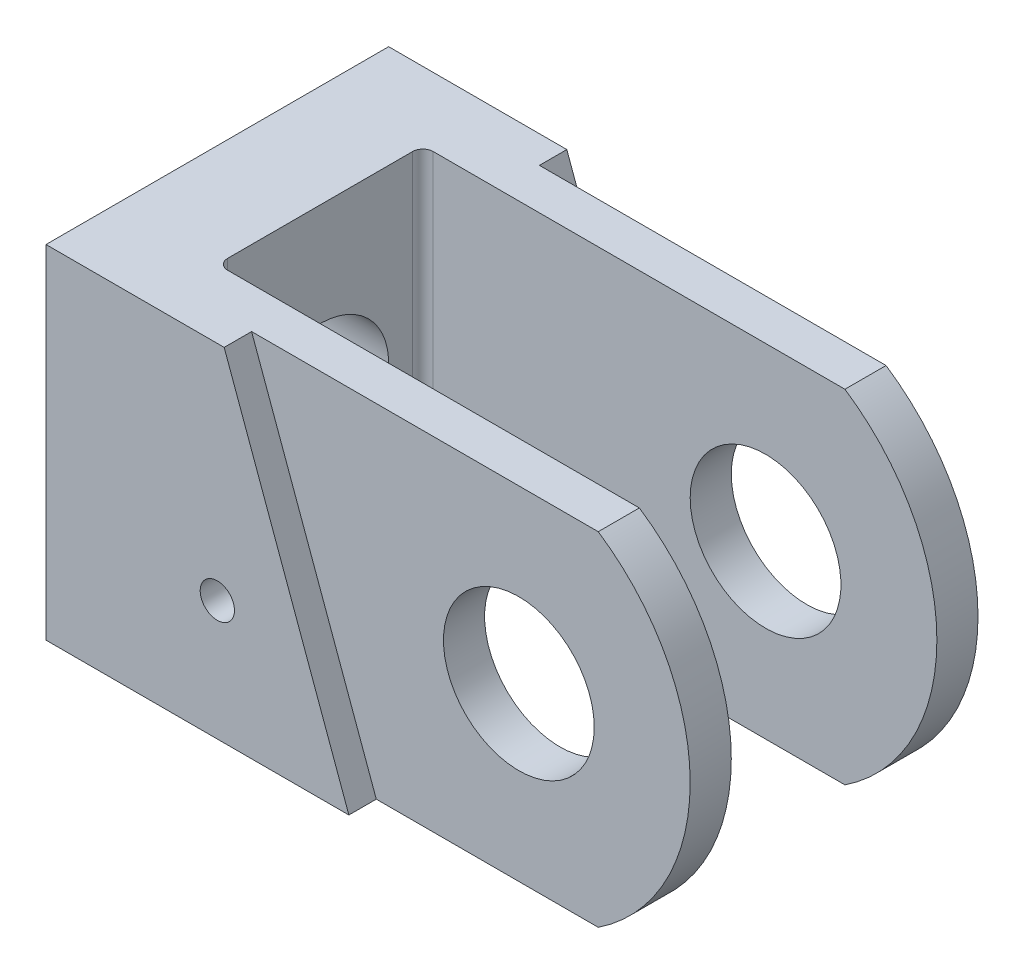
ISO-10303-21;
HEADER;
FILE_DESCRIPTION(('STEP AP214'),'2;1');
FILE_NAME('part.step','',(''),(''),'','','');
FILE_SCHEMA(('AUTOMOTIVE_DESIGN { 1 0 10303 214 1 1 1 1 }'));
ENDSEC;
DATA;
#1=APPLICATION_CONTEXT('core data for automotive mechanical design processes');
#2=APPLICATION_PROTOCOL_DEFINITION('international standard','automotive_design',2000,#1);
#3=PRODUCT_CONTEXT('',#1,'mechanical');
#4=PRODUCT('Part','Part','',(#3));
#5=PRODUCT_RELATED_PRODUCT_CATEGORY('part','',(#4));
#6=PRODUCT_DEFINITION_FORMATION('','',#4);
#7=PRODUCT_DEFINITION_CONTEXT('part definition',#1,'design');
#8=PRODUCT_DEFINITION('design','',#6,#7);
#9=PRODUCT_DEFINITION_SHAPE('','',#8);
#10=(LENGTH_UNIT() NAMED_UNIT(*) SI_UNIT(.MILLI.,.METRE.));
#11=(NAMED_UNIT(*) PLANE_ANGLE_UNIT() SI_UNIT($,.RADIAN.));
#12=(NAMED_UNIT(*) SI_UNIT($,.STERADIAN.) SOLID_ANGLE_UNIT());
#13=UNCERTAINTY_MEASURE_WITH_UNIT(LENGTH_MEASURE(1.E-05),#10,'distance_accuracy_value','');
#14=(GEOMETRIC_REPRESENTATION_CONTEXT(3) GLOBAL_UNCERTAINTY_ASSIGNED_CONTEXT((#13)) GLOBAL_UNIT_ASSIGNED_CONTEXT((#10,
#11,#12)) REPRESENTATION_CONTEXT('',''));
#15=CARTESIAN_POINT('',(0.,0.,0.));
#16=DIRECTION('',(0.,0.,1.));
#17=DIRECTION('',(1.,0.,0.));
#18=AXIS2_PLACEMENT_3D('',#15,#16,#17);
#19=CARTESIAN_POINT('',(-5.00000000000001,0.,25.));
#20=DIRECTION('',(0.,0.,-1.));
#21=DIRECTION('',(-1.,0.,0.));
#22=AXIS2_PLACEMENT_3D('',#19,#20,#21);
#23=CYLINDRICAL_SURFACE('',#22,30.);
#24=CARTESIAN_POINT('',(-5.00000000000001,0.,-21.));
#25=DIRECTION('',(0.,0.,1.));
#26=DIRECTION('',(1.,0.,0.));
#27=AXIS2_PLACEMENT_3D('',#24,#25,#26);
#28=CIRCLE('',#27,30.);
#29=CARTESIAN_POINT('',(11.583123951777,-25.,-21.));
#30=VERTEX_POINT('',#29);
#31=CARTESIAN_POINT('',(11.583123951777,25.,-21.));
#32=VERTEX_POINT('',#31);
#33=EDGE_CURVE('E145',#30,#32,#28,.T.);
#34=ORIENTED_EDGE('',*,*,#33,.T.);
#35=DIRECTION('',(0.,0.,-1.));
#36=VECTOR('',#35,1.);
#37=CARTESIAN_POINT('',(11.583123951777,25.,25.));
#38=LINE('',#37,#36);
#39=CARTESIAN_POINT('',(11.583123951777,25.,-15.));
#40=VERTEX_POINT('',#39);
#41=EDGE_CURVE('E154',#40,#32,#38,.T.);
#42=ORIENTED_EDGE('',*,*,#41,.F.);
#43=CARTESIAN_POINT('',(-5.00000000000001,0.,-15.));
#44=DIRECTION('',(0.,0.,-1.));
#45=DIRECTION('',(-1.,0.,0.));
#46=AXIS2_PLACEMENT_3D('',#43,#44,#45);
#47=CIRCLE('',#46,30.);
#48=CARTESIAN_POINT('',(11.583123951777,-25.,-15.));
#49=VERTEX_POINT('',#48);
#50=EDGE_CURVE('E238',#40,#49,#47,.T.);
#51=ORIENTED_EDGE('',*,*,#50,.T.);
#52=DIRECTION('',(0.,0.,-1.));
#53=VECTOR('',#52,1.);
#54=CARTESIAN_POINT('',(11.583123951777,-25.,25.));
#55=LINE('',#54,#53);
#56=EDGE_CURVE('E160',#49,#30,#55,.T.);
#57=ORIENTED_EDGE('',*,*,#56,.T.);
#58=EDGE_LOOP('',(#34,#42,#51,#57));
#59=FACE_BOUND('',#58,.T.);
#60=ADVANCED_FACE('F39',(#59),#23,.T.);
#61=CARTESIAN_POINT('',(0.,0.,25.));
#62=DIRECTION('',(0.,0.,-1.));
#63=DIRECTION('',(-1.,0.,0.));
#64=AXIS2_PLACEMENT_3D('',#61,#62,#63);
#65=CYLINDRICAL_SURFACE('',#64,11.);
#66=CARTESIAN_POINT('',(0.,0.,-15.));
#67=DIRECTION('',(0.,0.,-1.));
#68=DIRECTION('',(-1.,0.,0.));
#69=AXIS2_PLACEMENT_3D('',#66,#67,#68);
#70=CIRCLE('',#69,11.);
#71=CARTESIAN_POINT('',(-11.,0.,-15.));
#72=VERTEX_POINT('',#71);
#73=EDGE_CURVE('E186',#72,#72,#70,.T.);
#74=ORIENTED_EDGE('',*,*,#73,.F.);
#75=EDGE_LOOP('',(#74));
#76=FACE_BOUND('',#75,.T.);
#77=CARTESIAN_POINT('',(0.,0.,-21.));
#78=DIRECTION('',(0.,0.,-1.));
#79=DIRECTION('',(-1.,0.,0.));
#80=AXIS2_PLACEMENT_3D('',#77,#78,#79);
#81=CIRCLE('',#80,11.);
#82=CARTESIAN_POINT('',(-11.,0.,-21.));
#83=VERTEX_POINT('',#82);
#84=EDGE_CURVE('E294',#83,#83,#81,.T.);
#85=ORIENTED_EDGE('',*,*,#84,.T.);
#86=EDGE_LOOP('',(#85));
#87=FACE_BOUND('',#86,.T.);
#88=ADVANCED_FACE('F337',(#76,#87),#65,.F.);
#89=CARTESIAN_POINT('',(-5.00000000000001,0.,-25.));
#90=DIRECTION('',(0.,0.,-1.));
#91=DIRECTION('',(-1.,0.,0.));
#92=AXIS2_PLACEMENT_3D('',#89,#90,#91);
#93=PLANE('',#92);
#94=CARTESIAN_POINT('',(-40.,-7.5,-25.));
#95=DIRECTION('',(0.,0.,1.));
#96=DIRECTION('',(1.,0.,0.));
#97=AXIS2_PLACEMENT_3D('',#94,#95,#96);
#98=CIRCLE('',#97,2.5);
#99=CARTESIAN_POINT('',(-37.5,-7.5,-25.));
#100=VERTEX_POINT('',#99);
#101=EDGE_CURVE('E242',#100,#100,#98,.T.);
#102=ORIENTED_EDGE('',*,*,#101,.T.);
#103=EDGE_LOOP('',(#102));
#104=FACE_BOUND('',#103,.T.);
#105=DIRECTION('',(-1.,0.,0.));
#106=VECTOR('',#105,1.);
#107=CARTESIAN_POINT('',(-65.,25.,-25.));
#108=LINE('',#107,#106);
#109=CARTESIAN_POINT('',(-39.,25.,-25.));
#110=VERTEX_POINT('',#109);
#111=CARTESIAN_POINT('',(-65.,25.,-25.));
#112=VERTEX_POINT('',#111);
#113=EDGE_CURVE('E251',#110,#112,#108,.T.);
#114=ORIENTED_EDGE('',*,*,#113,.F.);
#115=DIRECTION('',(0.342020143325666,-0.939692620785909,0.));
#116=VECTOR('',#115,1.);
#117=CARTESIAN_POINT('',(-39.,25.,-25.));
#118=LINE('',#117,#116);
#119=CARTESIAN_POINT('',(-20.80148828669,-25.,-25.));
#120=VERTEX_POINT('',#119);
#121=EDGE_CURVE('E149',#110,#120,#118,.T.);
#122=ORIENTED_EDGE('',*,*,#121,.T.);
#123=DIRECTION('',(1.,0.,0.));
#124=VECTOR('',#123,1.);
#125=CARTESIAN_POINT('',(-65.,-25.,-25.));
#126=LINE('',#125,#124);
#127=CARTESIAN_POINT('',(-65.,-25.,-25.));
#128=VERTEX_POINT('',#127);
#129=EDGE_CURVE('E259',#128,#120,#126,.T.);
#130=ORIENTED_EDGE('',*,*,#129,.F.);
#131=DIRECTION('',(0.,-1.,0.));
#132=VECTOR('',#131,1.);
#133=CARTESIAN_POINT('',(-65.,25.,-25.));
#134=LINE('',#133,#132);
#135=EDGE_CURVE('E247',#112,#128,#134,.T.);
#136=ORIENTED_EDGE('',*,*,#135,.F.);
#137=EDGE_LOOP('',(#114,#122,#130,#136));
#138=FACE_BOUND('',#137,.T.);
#139=ADVANCED_FACE('F275',(#104,#138),#93,.T.);
#140=CARTESIAN_POINT('',(-65.,-25.,25.));
#141=DIRECTION('',(0.,1.,0.));
#142=DIRECTION('',(0.,0.,1.));
#143=AXIS2_PLACEMENT_3D('',#140,#141,#142);
#144=PLANE('',#143);
#145=DIRECTION('',(0.,0.,-1.));
#146=VECTOR('',#145,1.);
#147=CARTESIAN_POINT('',(-20.80148828669,-25.,-21.));
#148=LINE('',#147,#146);
#149=CARTESIAN_POINT('',(-20.80148828669,-25.,-21.));
#150=VERTEX_POINT('',#149);
#151=EDGE_CURVE('E303',#150,#120,#148,.T.);
#152=ORIENTED_EDGE('',*,*,#151,.F.);
#153=DIRECTION('',(1.,0.,0.));
#154=VECTOR('',#153,1.);
#155=CARTESIAN_POINT('',(-20.80148828669,-25.,-21.));
#156=LINE('',#155,#154);
#157=EDGE_CURVE('E158',#150,#30,#156,.T.);
#158=ORIENTED_EDGE('',*,*,#157,.T.);
#159=ORIENTED_EDGE('',*,*,#56,.F.);
#160=DIRECTION('',(-1.,0.,0.));
#161=VECTOR('',#160,1.);
#162=CARTESIAN_POINT('',(-50.,-25.,-15.));
#163=LINE('',#162,#161);
#164=CARTESIAN_POINT('',(-48.5,-25.,-15.));
#165=VERTEX_POINT('',#164);
#166=EDGE_CURVE('E185',#49,#165,#163,.T.);
#167=ORIENTED_EDGE('',*,*,#166,.T.);
#168=CARTESIAN_POINT('',(-48.5,-25.,-13.5));
#169=DIRECTION('',(0.,1.,0.));
#170=DIRECTION('',(0.,0.,1.));
#171=AXIS2_PLACEMENT_3D('',#168,#169,#170);
#172=CIRCLE('',#171,1.5);
#173=CARTESIAN_POINT('',(-50.,-25.,-13.5));
#174=VERTEX_POINT('',#173);
#175=EDGE_CURVE('E11',#165,#174,#172,.T.);
#176=ORIENTED_EDGE('',*,*,#175,.T.);
#177=DIRECTION('',(0.,0.,1.));
#178=VECTOR('',#177,1.);
#179=CARTESIAN_POINT('',(-50.,-25.,-15.));
#180=LINE('',#179,#178);
#181=CARTESIAN_POINT('',(-50.,-25.,13.5));
#182=VERTEX_POINT('',#181);
#183=EDGE_CURVE('E212',#174,#182,#180,.T.);
#184=ORIENTED_EDGE('',*,*,#183,.T.);
#185=CARTESIAN_POINT('',(-48.5,-25.,13.5));
#186=DIRECTION('',(0.,1.,0.));
#187=DIRECTION('',(0.,0.,1.));
#188=AXIS2_PLACEMENT_3D('',#185,#186,#187);
#189=CIRCLE('',#188,1.5);
#190=CARTESIAN_POINT('',(-48.5,-25.,15.));
#191=VERTEX_POINT('',#190);
#192=EDGE_CURVE('E201',#182,#191,#189,.T.);
#193=ORIENTED_EDGE('',*,*,#192,.T.);
#194=DIRECTION('',(1.,0.,0.));
#195=VECTOR('',#194,1.);
#196=CARTESIAN_POINT('',(-50.,-25.,15.));
#197=LINE('',#196,#195);
#198=CARTESIAN_POINT('',(11.583123951777,-25.,15.));
#199=VERTEX_POINT('',#198);
#200=EDGE_CURVE('E215',#191,#199,#197,.T.);
#201=ORIENTED_EDGE('',*,*,#200,.T.);
#202=CARTESIAN_POINT('',(11.583123951777,-25.,21.));
#203=VERTEX_POINT('',#202);
#204=EDGE_CURVE('E171',#203,#199,#55,.T.);
#205=ORIENTED_EDGE('',*,*,#204,.F.);
#206=DIRECTION('',(1.,0.,0.));
#207=VECTOR('',#206,1.);
#208=CARTESIAN_POINT('',(-20.80148828669,-25.,21.));
#209=LINE('',#208,#207);
#210=CARTESIAN_POINT('',(-20.80148828669,-25.,21.));
#211=VERTEX_POINT('',#210);
#212=EDGE_CURVE('E286',#211,#203,#209,.T.);
#213=ORIENTED_EDGE('',*,*,#212,.F.);
#214=DIRECTION('',(0.,0.,1.));
#215=VECTOR('',#214,1.);
#216=CARTESIAN_POINT('',(-20.80148828669,-25.,21.));
#217=LINE('',#216,#215);
#218=CARTESIAN_POINT('',(-20.80148828669,-25.,25.));
#219=VERTEX_POINT('',#218);
#220=EDGE_CURVE('E195',#211,#219,#217,.T.);
#221=ORIENTED_EDGE('',*,*,#220,.T.);
#222=DIRECTION('',(1.,0.,0.));
#223=VECTOR('',#222,1.);
#224=CARTESIAN_POINT('',(-65.,-25.,25.));
#225=LINE('',#224,#223);
#226=CARTESIAN_POINT('',(-65.,-25.,25.));
#227=VERTEX_POINT('',#226);
#228=EDGE_CURVE('E252',#227,#219,#225,.T.);
#229=ORIENTED_EDGE('',*,*,#228,.F.);
#230=DIRECTION('',(0.,0.,-1.));
#231=VECTOR('',#230,1.);
#232=CARTESIAN_POINT('',(-65.,-25.,25.));
#233=LINE('',#232,#231);
#234=EDGE_CURVE('E173',#227,#128,#233,.T.);
#235=ORIENTED_EDGE('',*,*,#234,.T.);
#236=ORIENTED_EDGE('',*,*,#129,.T.);
#237=EDGE_LOOP('',(#152,#158,#159,#167,#176,#184,#193,#201,#205,#213,#221,#229,#235,#236));
#238=FACE_BOUND('',#237,.T.);
#239=ADVANCED_FACE('F209',(#238),#144,.F.);
#240=CARTESIAN_POINT('',(-65.,25.,25.));
#241=DIRECTION('',(0.,-1.,0.));
#242=DIRECTION('',(0.,0.,-1.));
#243=AXIS2_PLACEMENT_3D('',#240,#241,#242);
#244=PLANE('',#243);
#245=DIRECTION('',(0.,0.,-1.));
#246=VECTOR('',#245,1.);
#247=CARTESIAN_POINT('',(-39.,25.,-21.));
#248=LINE('',#247,#246);
#249=CARTESIAN_POINT('',(-39.,25.,-21.));
#250=VERTEX_POINT('',#249);
#251=EDGE_CURVE('E264',#250,#110,#248,.T.);
#252=ORIENTED_EDGE('',*,*,#251,.T.);
#253=ORIENTED_EDGE('',*,*,#113,.T.);
#254=DIRECTION('',(0.,0.,-1.));
#255=VECTOR('',#254,1.);
#256=CARTESIAN_POINT('',(-65.,25.,25.));
#257=LINE('',#256,#255);
#258=CARTESIAN_POINT('',(-65.,25.,25.));
#259=VERTEX_POINT('',#258);
#260=EDGE_CURVE('E162',#259,#112,#257,.T.);
#261=ORIENTED_EDGE('',*,*,#260,.F.);
#262=DIRECTION('',(-1.,0.,0.));
#263=VECTOR('',#262,1.);
#264=CARTESIAN_POINT('',(-65.,25.,25.));
#265=LINE('',#264,#263);
#266=CARTESIAN_POINT('',(-39.,25.,25.));
#267=VERTEX_POINT('',#266);
#268=EDGE_CURVE('E170',#267,#259,#265,.T.);
#269=ORIENTED_EDGE('',*,*,#268,.F.);
#270=DIRECTION('',(0.,0.,1.));
#271=VECTOR('',#270,1.);
#272=CARTESIAN_POINT('',(-39.,25.,21.));
#273=LINE('',#272,#271);
#274=CARTESIAN_POINT('',(-39.,25.,21.));
#275=VERTEX_POINT('',#274);
#276=EDGE_CURVE('E282',#275,#267,#273,.T.);
#277=ORIENTED_EDGE('',*,*,#276,.F.);
#278=DIRECTION('',(-1.,0.,0.));
#279=VECTOR('',#278,1.);
#280=CARTESIAN_POINT('',(11.583123951777,25.,21.));
#281=LINE('',#280,#279);
#282=CARTESIAN_POINT('',(11.583123951777,25.,21.));
#283=VERTEX_POINT('',#282);
#284=EDGE_CURVE('E283',#283,#275,#281,.T.);
#285=ORIENTED_EDGE('',*,*,#284,.F.);
#286=CARTESIAN_POINT('',(11.583123951777,25.,15.));
#287=VERTEX_POINT('',#286);
#288=EDGE_CURVE('E165',#283,#287,#38,.T.);
#289=ORIENTED_EDGE('',*,*,#288,.T.);
#290=DIRECTION('',(1.,0.,0.));
#291=VECTOR('',#290,1.);
#292=CARTESIAN_POINT('',(-50.,25.,15.));
#293=LINE('',#292,#291);
#294=CARTESIAN_POINT('',(-48.5,25.,15.));
#295=VERTEX_POINT('',#294);
#296=EDGE_CURVE('E226',#295,#287,#293,.T.);
#297=ORIENTED_EDGE('',*,*,#296,.F.);
#298=CARTESIAN_POINT('',(-48.5,25.,13.5));
#299=DIRECTION('',(0.,-1.,0.));
#300=DIRECTION('',(0.,0.,-1.));
#301=AXIS2_PLACEMENT_3D('',#298,#299,#300);
#302=CIRCLE('',#301,1.5);
#303=CARTESIAN_POINT('',(-50.,25.,13.5));
#304=VERTEX_POINT('',#303);
#305=EDGE_CURVE('E203',#295,#304,#302,.T.);
#306=ORIENTED_EDGE('',*,*,#305,.T.);
#307=DIRECTION('',(0.,0.,1.));
#308=VECTOR('',#307,1.);
#309=CARTESIAN_POINT('',(-50.,25.,-15.));
#310=LINE('',#309,#308);
#311=CARTESIAN_POINT('',(-50.,25.,-13.5));
#312=VERTEX_POINT('',#311);
#313=EDGE_CURVE('E192',#312,#304,#310,.T.);
#314=ORIENTED_EDGE('',*,*,#313,.F.);
#315=CARTESIAN_POINT('',(-48.5,25.,-13.5));
#316=DIRECTION('',(0.,-1.,0.));
#317=DIRECTION('',(0.,0.,-1.));
#318=AXIS2_PLACEMENT_3D('',#315,#316,#317);
#319=CIRCLE('',#318,1.5);
#320=CARTESIAN_POINT('',(-48.5,25.,-15.));
#321=VERTEX_POINT('',#320);
#322=EDGE_CURVE('E48',#312,#321,#319,.T.);
#323=ORIENTED_EDGE('',*,*,#322,.T.);
#324=DIRECTION('',(-1.,0.,0.));
#325=VECTOR('',#324,1.);
#326=CARTESIAN_POINT('',(-50.,25.,-15.));
#327=LINE('',#326,#325);
#328=EDGE_CURVE('E161',#40,#321,#327,.T.);
#329=ORIENTED_EDGE('',*,*,#328,.F.);
#330=ORIENTED_EDGE('',*,*,#41,.T.);
#331=DIRECTION('',(-1.,0.,0.));
#332=VECTOR('',#331,1.);
#333=CARTESIAN_POINT('',(11.583123951777,25.,-21.));
#334=LINE('',#333,#332);
#335=EDGE_CURVE('E136',#32,#250,#334,.T.);
#336=ORIENTED_EDGE('',*,*,#335,.T.);
#337=EDGE_LOOP('',(#252,#253,#261,#269,#277,#285,#289,#297,#306,#314,#323,#329,#330,#336));
#338=FACE_BOUND('',#337,.T.);
#339=ADVANCED_FACE('F159',(#338),#244,.F.);
#340=CARTESIAN_POINT('',(-5.00000000000001,0.,21.));
#341=DIRECTION('',(0.,0.,1.));
#342=DIRECTION('',(1.,0.,0.));
#343=AXIS2_PLACEMENT_3D('',#340,#341,#342);
#344=CIRCLE('',#343,30.);
#345=EDGE_CURVE('E290',#203,#283,#344,.T.);
#346=ORIENTED_EDGE('',*,*,#345,.F.);
#347=ORIENTED_EDGE('',*,*,#204,.T.);
#348=CARTESIAN_POINT('',(-5.00000000000001,0.,15.));
#349=DIRECTION('',(0.,0.,1.));
#350=DIRECTION('',(1.,0.,0.));
#351=AXIS2_PLACEMENT_3D('',#348,#349,#350);
#352=CIRCLE('',#351,30.);
#353=EDGE_CURVE('E187',#199,#287,#352,.T.);
#354=ORIENTED_EDGE('',*,*,#353,.T.);
#355=ORIENTED_EDGE('',*,*,#288,.F.);
#356=EDGE_LOOP('',(#346,#347,#354,#355));
#357=FACE_BOUND('',#356,.T.);
#358=ADVANCED_FACE('F338',(#357),#23,.T.);
#359=CARTESIAN_POINT('',(0.,0.,15.));
#360=DIRECTION('',(0.,0.,1.));
#361=DIRECTION('',(1.,0.,0.));
#362=AXIS2_PLACEMENT_3D('',#359,#360,#361);
#363=CIRCLE('',#362,11.);
#364=CARTESIAN_POINT('',(11.,0.,15.));
#365=VERTEX_POINT('',#364);
#366=EDGE_CURVE('E182',#365,#365,#363,.T.);
#367=ORIENTED_EDGE('',*,*,#366,.F.);
#368=EDGE_LOOP('',(#367));
#369=FACE_BOUND('',#368,.T.);
#370=CARTESIAN_POINT('',(0.,0.,21.));
#371=DIRECTION('',(0.,0.,1.));
#372=DIRECTION('',(1.,0.,0.));
#373=AXIS2_PLACEMENT_3D('',#370,#371,#372);
#374=CIRCLE('',#373,11.);
#375=CARTESIAN_POINT('',(11.,0.,21.));
#376=VERTEX_POINT('',#375);
#377=EDGE_CURVE('E189',#376,#376,#374,.T.);
#378=ORIENTED_EDGE('',*,*,#377,.T.);
#379=EDGE_LOOP('',(#378));
#380=FACE_BOUND('',#379,.T.);
#381=ADVANCED_FACE('F347',(#369,#380),#65,.F.);
#382=CARTESIAN_POINT('',(-40.,-7.5,25.));
#383=DIRECTION('',(0.,0.,-1.));
#384=DIRECTION('',(-1.,0.,0.));
#385=AXIS2_PLACEMENT_3D('',#382,#383,#384);
#386=CYLINDRICAL_SURFACE('',#385,2.5);
#387=CARTESIAN_POINT('',(-40.,-7.5,-15.));
#388=DIRECTION('',(0.,0.,-1.));
#389=DIRECTION('',(-1.,0.,0.));
#390=AXIS2_PLACEMENT_3D('',#387,#388,#389);
#391=CIRCLE('',#390,2.5);
#392=CARTESIAN_POINT('',(-42.5,-7.5,-15.));
#393=VERTEX_POINT('',#392);
#394=EDGE_CURVE('E181',#393,#393,#391,.T.);
#395=ORIENTED_EDGE('',*,*,#394,.F.);
#396=EDGE_LOOP('',(#395));
#397=FACE_BOUND('',#396,.T.);
#398=ORIENTED_EDGE('',*,*,#101,.F.);
#399=EDGE_LOOP('',(#398));
#400=FACE_BOUND('',#399,.T.);
#401=ADVANCED_FACE('F335',(#397,#400),#386,.F.);
#402=CARTESIAN_POINT('',(-5.00000000000001,0.,25.));
#403=DIRECTION('',(0.,0.,-1.));
#404=DIRECTION('',(-1.,0.,0.));
#405=AXIS2_PLACEMENT_3D('',#402,#403,#404);
#406=PLANE('',#405);
#407=ORIENTED_EDGE('',*,*,#228,.T.);
#408=DIRECTION('',(0.342020143325666,-0.939692620785909,0.));
#409=VECTOR('',#408,1.);
#410=CARTESIAN_POINT('',(-39.,25.,25.));
#411=LINE('',#410,#409);
#412=EDGE_CURVE('E276',#267,#219,#411,.T.);
#413=ORIENTED_EDGE('',*,*,#412,.F.);
#414=ORIENTED_EDGE('',*,*,#268,.T.);
#415=DIRECTION('',(0.,-1.,0.));
#416=VECTOR('',#415,1.);
#417=CARTESIAN_POINT('',(-65.,25.,25.));
#418=LINE('',#417,#416);
#419=EDGE_CURVE('E249',#259,#227,#418,.T.);
#420=ORIENTED_EDGE('',*,*,#419,.T.);
#421=EDGE_LOOP('',(#407,#413,#414,#420));
#422=FACE_BOUND('',#421,.T.);
#423=CARTESIAN_POINT('',(-40.,-7.5,25.));
#424=DIRECTION('',(0.,0.,1.));
#425=DIRECTION('',(1.,0.,0.));
#426=AXIS2_PLACEMENT_3D('',#423,#424,#425);
#427=CIRCLE('',#426,2.5);
#428=CARTESIAN_POINT('',(-37.5,-7.5,25.));
#429=VERTEX_POINT('',#428);
#430=EDGE_CURVE('E244',#429,#429,#427,.T.);
#431=ORIENTED_EDGE('',*,*,#430,.F.);
#432=EDGE_LOOP('',(#431));
#433=FACE_BOUND('',#432,.T.);
#434=ADVANCED_FACE('F280',(#422,#433),#406,.F.);
#435=CARTESIAN_POINT('',(-65.,25.,25.));
#436=DIRECTION('',(1.,0.,0.));
#437=DIRECTION('',(0.,1.,0.));
#438=AXIS2_PLACEMENT_3D('',#435,#436,#437);
#439=PLANE('',#438);
#440=CARTESIAN_POINT('',(-65.,0.,0.));
#441=DIRECTION('',(-1.,0.,0.));
#442=DIRECTION('',(0.,0.,1.));
#443=AXIS2_PLACEMENT_3D('',#440,#441,#442);
#444=CIRCLE('',#443,17.5);
#445=CARTESIAN_POINT('',(-65.,0.,17.5));
#446=VERTEX_POINT('',#445);
#447=EDGE_CURVE('E312',#446,#446,#444,.T.);
#448=ORIENTED_EDGE('',*,*,#447,.F.);
#449=EDGE_LOOP('',(#448));
#450=FACE_BOUND('',#449,.T.);
#451=ORIENTED_EDGE('',*,*,#135,.T.);
#452=ORIENTED_EDGE('',*,*,#234,.F.);
#453=ORIENTED_EDGE('',*,*,#419,.F.);
#454=ORIENTED_EDGE('',*,*,#260,.T.);
#455=EDGE_LOOP('',(#451,#452,#453,#454));
#456=FACE_BOUND('',#455,.T.);
#457=ADVANCED_FACE('F269',(#450,#456),#439,.F.);
#458=CARTESIAN_POINT('',(-40.,-7.5,15.));
#459=DIRECTION('',(0.,0.,1.));
#460=DIRECTION('',(1.,0.,0.));
#461=AXIS2_PLACEMENT_3D('',#458,#459,#460);
#462=CIRCLE('',#461,2.5);
#463=CARTESIAN_POINT('',(-37.5,-7.5,15.));
#464=VERTEX_POINT('',#463);
#465=EDGE_CURVE('E178',#464,#464,#462,.T.);
#466=ORIENTED_EDGE('',*,*,#465,.F.);
#467=EDGE_LOOP('',(#466));
#468=FACE_BOUND('',#467,.T.);
#469=ORIENTED_EDGE('',*,*,#430,.T.);
#470=EDGE_LOOP('',(#469));
#471=FACE_BOUND('',#470,.T.);
#472=ADVANCED_FACE('F325',(#468,#471),#386,.F.);
#473=CARTESIAN_POINT('',(-50.,-25.,-15.));
#474=DIRECTION('',(0.,0.,-1.));
#475=DIRECTION('',(-1.,0.,0.));
#476=AXIS2_PLACEMENT_3D('',#473,#474,#475);
#477=PLANE('',#476);
#478=ORIENTED_EDGE('',*,*,#73,.T.);
#479=EDGE_LOOP('',(#478));
#480=FACE_BOUND('',#479,.T.);
#481=ORIENTED_EDGE('',*,*,#394,.T.);
#482=EDGE_LOOP('',(#481));
#483=FACE_BOUND('',#482,.T.);
#484=ORIENTED_EDGE('',*,*,#328,.T.);
#485=DIRECTION('',(0.,1.,0.));
#486=VECTOR('',#485,1.);
#487=CARTESIAN_POINT('',(-48.5,-25.,-15.));
#488=LINE('',#487,#486);
#489=EDGE_CURVE('E54',#321,#165,#488,.F.);
#490=ORIENTED_EDGE('',*,*,#489,.T.);
#491=ORIENTED_EDGE('',*,*,#166,.F.);
#492=ORIENTED_EDGE('',*,*,#50,.F.);
#493=EDGE_LOOP('',(#484,#490,#491,#492));
#494=FACE_BOUND('',#493,.T.);
#495=ADVANCED_FACE('F328',(#480,#483,#494),#477,.F.);
#496=CARTESIAN_POINT('',(-50.,-25.,15.));
#497=DIRECTION('',(0.,0.,1.));
#498=DIRECTION('',(1.,0.,0.));
#499=AXIS2_PLACEMENT_3D('',#496,#497,#498);
#500=PLANE('',#499);
#501=ORIENTED_EDGE('',*,*,#366,.T.);
#502=EDGE_LOOP('',(#501));
#503=FACE_BOUND('',#502,.T.);
#504=ORIENTED_EDGE('',*,*,#465,.T.);
#505=EDGE_LOOP('',(#504));
#506=FACE_BOUND('',#505,.T.);
#507=ORIENTED_EDGE('',*,*,#200,.F.);
#508=DIRECTION('',(0.,1.,0.));
#509=VECTOR('',#508,1.);
#510=CARTESIAN_POINT('',(-48.5,25.,15.));
#511=LINE('',#510,#509);
#512=EDGE_CURVE('E180',#191,#295,#511,.T.);
#513=ORIENTED_EDGE('',*,*,#512,.T.);
#514=ORIENTED_EDGE('',*,*,#296,.T.);
#515=ORIENTED_EDGE('',*,*,#353,.F.);
#516=EDGE_LOOP('',(#507,#513,#514,#515));
#517=FACE_BOUND('',#516,.T.);
#518=ADVANCED_FACE('F219',(#503,#506,#517),#500,.F.);
#519=CARTESIAN_POINT('',(-50.,-25.,-15.));
#520=DIRECTION('',(-1.,0.,0.));
#521=DIRECTION('',(0.,0.,1.));
#522=AXIS2_PLACEMENT_3D('',#519,#520,#521);
#523=PLANE('',#522);
#524=CARTESIAN_POINT('',(-50.,0.,0.));
#525=DIRECTION('',(-1.,0.,0.));
#526=DIRECTION('',(0.,0.,1.));
#527=AXIS2_PLACEMENT_3D('',#524,#525,#526);
#528=CIRCLE('',#527,10.);
#529=CARTESIAN_POINT('',(-50.,0.,10.));
#530=VERTEX_POINT('',#529);
#531=EDGE_CURVE('E43',#530,#530,#528,.T.);
#532=ORIENTED_EDGE('',*,*,#531,.T.);
#533=EDGE_LOOP('',(#532));
#534=FACE_BOUND('',#533,.T.);
#535=ORIENTED_EDGE('',*,*,#313,.T.);
#536=DIRECTION('',(0.,1.,0.));
#537=VECTOR('',#536,1.);
#538=CARTESIAN_POINT('',(-50.,-25.,13.5));
#539=LINE('',#538,#537);
#540=EDGE_CURVE('E196',#304,#182,#539,.F.);
#541=ORIENTED_EDGE('',*,*,#540,.T.);
#542=ORIENTED_EDGE('',*,*,#183,.F.);
#543=DIRECTION('',(0.,1.,0.));
#544=VECTOR('',#543,1.);
#545=CARTESIAN_POINT('',(-50.,25.,-13.5));
#546=LINE('',#545,#544);
#547=EDGE_CURVE('E191',#174,#312,#546,.T.);
#548=ORIENTED_EDGE('',*,*,#547,.T.);
#549=EDGE_LOOP('',(#535,#541,#542,#548));
#550=FACE_BOUND('',#549,.T.);
#551=ADVANCED_FACE('F229',(#534,#550),#523,.F.);
#552=CARTESIAN_POINT('',(-39.,25.,21.));
#553=DIRECTION('',(-0.939692620785909,-0.342020143325666,0.));
#554=DIRECTION('',(0.342020143325666,-0.939692620785909,0.));
#555=AXIS2_PLACEMENT_3D('',#552,#553,#554);
#556=PLANE('',#555);
#557=ORIENTED_EDGE('',*,*,#412,.T.);
#558=ORIENTED_EDGE('',*,*,#220,.F.);
#559=DIRECTION('',(0.342020143325666,-0.939692620785909,0.));
#560=VECTOR('',#559,1.);
#561=CARTESIAN_POINT('',(-39.,25.,21.));
#562=LINE('',#561,#560);
#563=EDGE_CURVE('E297',#275,#211,#562,.T.);
#564=ORIENTED_EDGE('',*,*,#563,.F.);
#565=ORIENTED_EDGE('',*,*,#276,.T.);
#566=EDGE_LOOP('',(#557,#558,#564,#565));
#567=FACE_BOUND('',#566,.T.);
#568=ADVANCED_FACE('F358',(#567),#556,.F.);
#569=CARTESIAN_POINT('',(-5.00000000000001,0.,21.));
#570=DIRECTION('',(0.,0.,1.));
#571=DIRECTION('',(1.,0.,0.));
#572=AXIS2_PLACEMENT_3D('',#569,#570,#571);
#573=PLANE('',#572);
#574=ORIENTED_EDGE('',*,*,#377,.F.);
#575=EDGE_LOOP('',(#574));
#576=FACE_BOUND('',#575,.T.);
#577=ORIENTED_EDGE('',*,*,#284,.T.);
#578=ORIENTED_EDGE('',*,*,#563,.T.);
#579=ORIENTED_EDGE('',*,*,#212,.T.);
#580=ORIENTED_EDGE('',*,*,#345,.T.);
#581=EDGE_LOOP('',(#577,#578,#579,#580));
#582=FACE_BOUND('',#581,.T.);
#583=ADVANCED_FACE('F360',(#576,#582),#573,.T.);
#584=CARTESIAN_POINT('',(-39.,25.,-21.));
#585=DIRECTION('',(0.939692620785909,0.342020143325666,0.));
#586=DIRECTION('',(-0.342020143325666,0.939692620785909,0.));
#587=AXIS2_PLACEMENT_3D('',#584,#585,#586);
#588=PLANE('',#587);
#589=ORIENTED_EDGE('',*,*,#121,.F.);
#590=ORIENTED_EDGE('',*,*,#251,.F.);
#591=DIRECTION('',(0.342020143325666,-0.939692620785909,0.));
#592=VECTOR('',#591,1.);
#593=CARTESIAN_POINT('',(-39.,25.,-21.));
#594=LINE('',#593,#592);
#595=EDGE_CURVE('E148',#250,#150,#594,.T.);
#596=ORIENTED_EDGE('',*,*,#595,.T.);
#597=ORIENTED_EDGE('',*,*,#151,.T.);
#598=EDGE_LOOP('',(#589,#590,#596,#597));
#599=FACE_BOUND('',#598,.T.);
#600=ADVANCED_FACE('F361',(#599),#588,.T.);
#601=CARTESIAN_POINT('',(-5.00000000000001,0.,-21.));
#602=DIRECTION('',(0.,0.,-1.));
#603=DIRECTION('',(1.,0.,0.));
#604=AXIS2_PLACEMENT_3D('',#601,#602,#603);
#605=PLANE('',#604);
#606=ORIENTED_EDGE('',*,*,#84,.F.);
#607=EDGE_LOOP('',(#606));
#608=FACE_BOUND('',#607,.T.);
#609=ORIENTED_EDGE('',*,*,#335,.F.);
#610=ORIENTED_EDGE('',*,*,#33,.F.);
#611=ORIENTED_EDGE('',*,*,#157,.F.);
#612=ORIENTED_EDGE('',*,*,#595,.F.);
#613=EDGE_LOOP('',(#609,#610,#611,#612));
#614=FACE_BOUND('',#613,.T.);
#615=ADVANCED_FACE('F142',(#608,#614),#605,.T.);
#616=CARTESIAN_POINT('',(-48.5,-25.,13.5));
#617=DIRECTION('',(0.,-1.,0.));
#618=DIRECTION('',(0.,0.,-1.));
#619=AXIS2_PLACEMENT_3D('',#616,#617,#618);
#620=CYLINDRICAL_SURFACE('',#619,1.5);
#621=ORIENTED_EDGE('',*,*,#192,.F.);
#622=ORIENTED_EDGE('',*,*,#540,.F.);
#623=ORIENTED_EDGE('',*,*,#305,.F.);
#624=ORIENTED_EDGE('',*,*,#512,.F.);
#625=EDGE_LOOP('',(#621,#622,#623,#624));
#626=FACE_BOUND('',#625,.T.);
#627=ADVANCED_FACE('F221',(#626),#620,.F.);
#628=CARTESIAN_POINT('',(-48.5,-25.,-13.5));
#629=DIRECTION('',(0.,-1.,0.));
#630=DIRECTION('',(0.,0.,-1.));
#631=AXIS2_PLACEMENT_3D('',#628,#629,#630);
#632=CYLINDRICAL_SURFACE('',#631,1.5);
#633=ORIENTED_EDGE('',*,*,#175,.F.);
#634=ORIENTED_EDGE('',*,*,#489,.F.);
#635=ORIENTED_EDGE('',*,*,#322,.F.);
#636=ORIENTED_EDGE('',*,*,#547,.F.);
#637=EDGE_LOOP('',(#633,#634,#635,#636));
#638=FACE_BOUND('',#637,.T.);
#639=ADVANCED_FACE('F41',(#638),#632,.F.);
#640=CARTESIAN_POINT('',(-65.,0.,0.));
#641=DIRECTION('',(-1.,0.,0.));
#642=DIRECTION('',(0.,0.,1.));
#643=AXIS2_PLACEMENT_3D('',#640,#641,#642);
#644=CYLINDRICAL_SURFACE('',#643,10.);
#645=CARTESIAN_POINT('',(-63.,0.,0.));
#646=DIRECTION('',(-1.,0.,0.));
#647=DIRECTION('',(0.,0.,1.));
#648=AXIS2_PLACEMENT_3D('',#645,#646,#647);
#649=CIRCLE('',#648,10.);
#650=CARTESIAN_POINT('',(-63.,0.,10.));
#651=VERTEX_POINT('',#650);
#652=EDGE_CURVE('E310',#651,#651,#649,.T.);
#653=ORIENTED_EDGE('',*,*,#652,.T.);
#654=EDGE_LOOP('',(#653));
#655=FACE_BOUND('',#654,.T.);
#656=ORIENTED_EDGE('',*,*,#531,.F.);
#657=EDGE_LOOP('',(#656));
#658=FACE_BOUND('',#657,.T.);
#659=ADVANCED_FACE('F399',(#655,#658),#644,.F.);
#660=CARTESIAN_POINT('',(-63.,10.,0.));
#661=DIRECTION('',(1.,0.,0.));
#662=DIRECTION('',(0.,0.,-1.));
#663=AXIS2_PLACEMENT_3D('',#660,#661,#662);
#664=PLANE('',#663);
#665=ORIENTED_EDGE('',*,*,#652,.F.);
#666=EDGE_LOOP('',(#665));
#667=FACE_BOUND('',#666,.T.);
#668=CARTESIAN_POINT('',(-63.,0.,0.));
#669=DIRECTION('',(-1.,0.,0.));
#670=DIRECTION('',(0.,0.,1.));
#671=AXIS2_PLACEMENT_3D('',#668,#669,#670);
#672=CIRCLE('',#671,17.5);
#673=CARTESIAN_POINT('',(-63.,0.,17.5));
#674=VERTEX_POINT('',#673);
#675=EDGE_CURVE('E315',#674,#674,#672,.T.);
#676=ORIENTED_EDGE('',*,*,#675,.T.);
#677=EDGE_LOOP('',(#676));
#678=FACE_BOUND('',#677,.T.);
#679=ADVANCED_FACE('F405',(#667,#678),#664,.F.);
#680=CARTESIAN_POINT('',(-65.,0.,0.));
#681=DIRECTION('',(-1.,0.,0.));
#682=DIRECTION('',(0.,0.,1.));
#683=AXIS2_PLACEMENT_3D('',#680,#681,#682);
#684=CYLINDRICAL_SURFACE('',#683,17.5);
#685=ORIENTED_EDGE('',*,*,#675,.F.);
#686=EDGE_LOOP('',(#685));
#687=FACE_BOUND('',#686,.T.);
#688=ORIENTED_EDGE('',*,*,#447,.T.);
#689=EDGE_LOOP('',(#688));
#690=FACE_BOUND('',#689,.T.);
#691=ADVANCED_FACE('F317',(#687,#690),#684,.F.);
#692=CLOSED_SHELL('',(#60,#88,#139,#239,#339,#358,#381,#401,#434,#457,#472,#495,#518,#551,#568,
#583,#600,#615,#627,#639,#659,#679,#691));
#693=MANIFOLD_SOLID_BREP('B2',#692);
#694=ADVANCED_BREP_SHAPE_REPRESENTATION('',(#18,#693),#14);
#695=SHAPE_DEFINITION_REPRESENTATION(#9,#694);
ENDSEC;
END-ISO-10303-21;
